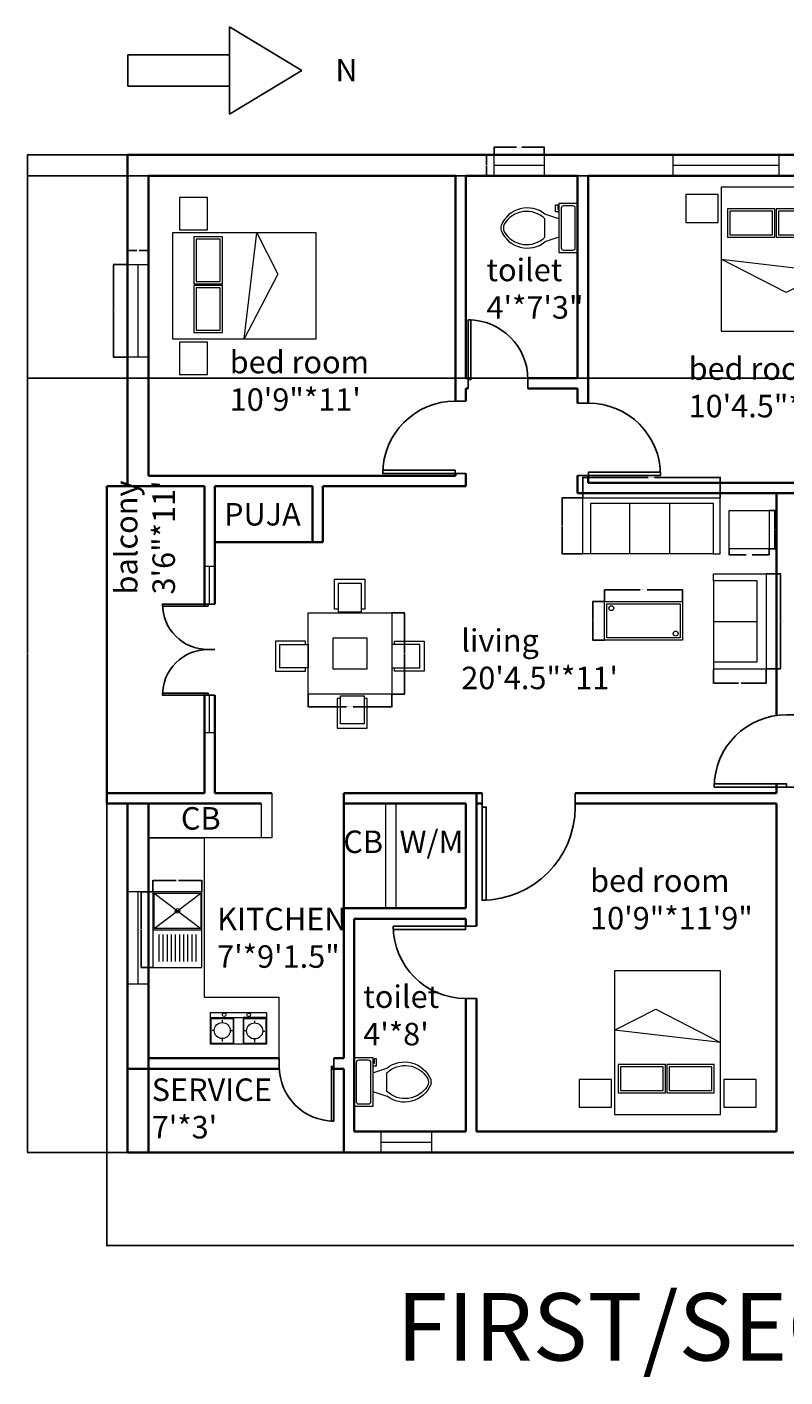
# Model space of a CAD drawing. Units: inches. Extents: x 1632 to 2336, y 1480 to 2095.
# Tile 1 of 2: x 1632 to 1958, y 1480 to 2061. Entities that reach past the tile are written whole.
import ezdxf

# ---------------------------------------------------------------- set-up
doc = ezdxf.new("R2010")
doc.units = ezdxf.units.IN
for name, color, linetype, lineweight in [('A-ANNO-DIMS', 2, 'Continuous', 18), ('A-ANNO-SYMB', 7, 'Continuous', 25), ('A-ANNO-TEXT', 7, 'Continuous', 18), ('A-ANNO-TITL', 7, 'Continuous', 35), ('A-AREA-IDEN', 7, 'Continuous', 18), ('A-DOOR', 3, 'Continuous', 25), ('A-EQPM', 8, 'Continuous', 18), ('A-FLOR-CASE', 9, 'Continuous', 18), ('A-FLOR-FIXT', 9, 'Continuous', 18), ('A-FURN', 8, 'Continuous', 18), ('A-GLAZ', 4, 'Continuous', 18), ('A-WALL', 7, 'Continuous', 35)]:
    doc.layers.add(name, color=color, linetype=linetype, lineweight=lineweight)
doc.styles.get("Standard").update_dxf_attribs({"font": 'arial.ttf'})
doc.dimstyles.get("Standard").update_dxf_attribs({"dimtxt": 0.18, "dimasz": 0.18, "dimexe": 0.18, "dimexo": 0.0625, "dimgap": 0.09, "dimtad": 0, "dimtih": 1, "dimtoh": 1, "dimdec": 4, "dimzin": 0, "dimdsep": 46, "dimtxsty": 'Standard', "dimcen": 0.09, "dimadec": 0, "dimazin": 0, "dimtfac": 1, "dimtdec": 4, "dimtofl": 0, "dimtmove": 0, "dimatfit": 3, "dimfxl": 1, "dimtolj": 1, "dimtzin": 0, "dimarcsym": 0})

# ---------------------------------------------------------------- blocks, each defined once
blk = doc.blocks.new('*U2')
for p, q in [((0, 0), (0, -6)), ((40, 0), (40, -6))]:
    blk.add_line(p, q)
blk.add_lwpolyline([(0, 0), (0, 40), (1.75, 40), (1.75, 0)], close=True)
blk.add_arc((0, 0), 40, 0, 90)
blk = doc.blocks.new('*U4')
for p, q in [((9.5, -6), (9.5, -2)), ((-10, -8.5), (-8, -8.5)), ((-10, -9.5), (-10, -8.5)), ((-7, -9.5), (-10, -9.5)), ((-8, -8.5), (-8, -8)), ((-7, -8), (-7, -9.5)), ((-4, -8), (-6, -14)), ((4, -8), (6, -14)), ((4, -14), (-4, -14))]:
    blk.add_line(p, q)
blk.add_lwpolyline([(10.5, -8), (10.5, 0), (-10.5, 0), (-10.5, -8)], close=True)
for points in [[(-9.5, -2), (-9.5, -6)], [(8.5, -1), (-8.5, -1)], [(-8.5, -7), (8.5, -7)]]:
    blk.add_lwpolyline(points)
for centre, radius, start, end in [((-8.62, -1.88), 0.884, 81.8699, 188.1301), ((8.62, -1.88), 0.884, 351.8699, 98.1301), ((-8.62, -6.12), 0.884, 171.8699, 278.1301), ((8.62, -6.12), 0.884, 261.8699, 8.1301), ((3.52, -21.58), 12.17, 141.46911, 247.97143), ((4.2, -21.82), 11.33, 136.36773, 238.94682), ((-3.52, -21.58), 12.17, 292.02843, 38.53071), ((-4.2, -21.82), 11.33, 301.05301, 43.63209), ((0, -27.88), 4, 245.73182, 294.26817), ((0, -29), 4, 254.86053, 285.13947)]:
    blk.add_arc(centre, radius, start, end)
blk = doc.blocks.new('BED-DOUBLE-WITH-NIGHTSTANDS')
for p, q in [((30.9, 15.3), (36.28, 60.91)), ((36.28, 60.91), (45.27, 43.14)), ((45.27, 43.14), (30.9, 15.3))]:
    blk.add_line(p, q)
for points in [[(3.09, 62.18), (15.1, 62.18), (15.1, 76.08), (3.09, 76.08)], [(0, 15.3), (61.8, 15.3), (61.8, 60.91), (0, 60.91)], [(9.26, 38.94), (21.51, 38.94), (21.51, 59.23), (9.26, 59.23)], [(10.26, 39.94), (20.51, 39.94), (20.51, 58.23), (10.26, 58.23)], [(9.26, 18.02), (21.51, 18.02), (21.51, 38.31), (9.26, 38.31)], [(10.26, 19.02), (20.51, 19.02), (20.51, 37.31), (10.26, 37.31)], [(3.09, 0), (15.1, 0), (15.1, 13.9), (3.09, 13.9)]]:
    blk.add_lwpolyline(points, close=True)
blk = doc.blocks.new('CHAIR-DINING')
for p, q in [((0, 1.12), (0, 13.97)), ((0, 13.97), (12.95, 13.97)), ((12.95, 13.97), (12.95, 1.12)), ((1.47, 1.12), (0, 1.12)), ((12.95, 1.12), (11.55, 1.12))]:
    blk.add_line(p, q)
blk.add_lwpolyline([(1.47, 0), (11.55, 0), (11.55, 12.08), (1.47, 12.08)], close=True)
blk = doc.blocks.new('TABLE-DINING')
for points in [[(0, 35.03), (36, 35.03), (36, 0), (0, 0)], [(10.77, 24.25), (25.23, 24.25), (25.23, 10.77), (10.77, 10.77)]]:
    blk.add_lwpolyline(points, close=True)
blk = doc.blocks.new('SOFA-3-SEAT')
for p, q in [((0, 0), (0, 24.07)), ((0, 24.07), (59, 24.07)), ((59, 0), (59, 24.07)), ((20.13, 21.83), (20.13, 0)), ((37.25, 21.83), (37.25, 0)), ((3.41, 0), (0, 0)), ((56, 0), (59, 0))]:
    blk.add_line(p, q)
blk.add_lwpolyline([(3.41, 21.83), (56, 21.83), (56, 0), (3.41, 0)], close=True)
blk = doc.blocks.new('SOFA-2-SEAT')
for p, q in [((0, 37.84), (0, 40.84)), ((0, 40.84), (22.7, 40.84)), ((22.7, 40.84), (22.7, 0)), ((0, 20.42), (18.79, 20.42)), ((0, 3), (0, 0)), ((0, 0), (22.7, 0))]:
    blk.add_line(p, q)
blk.add_lwpolyline([(18.79, 37.84), (0, 37.84), (0, 3), (18.79, 3)], close=True)
blk = doc.blocks.new('TABLE-COFFEE')
for points in [[(0, 16.65), (33.49, 16.65), (33.49, 0), (0, 0)], [(1, 15.65), (32.49, 15.65), (32.49, 1), (1, 1)]]:
    blk.add_lwpolyline(points, close=True)
for centre in [(2.89, 13.8), (30.54, 2.86)]:
    blk.add_circle(centre, 1.06)
blk = doc.blocks.new('SINK-WITH-DRAINBOARD')
for p, q in [((0.63, 16.78), (20.68, 31.97)), ((0.63, 31.97), (20.68, 16.78)), ((0, 16.25), (21.16, 16.25)), ((2.61, 14.26), (2.61, 2.54)), ((4.39, 14.26), (4.39, 2.54)), ((6.16, 14.26), (6.16, 2.54)), ((7.94, 14.26), (7.94, 2.54)), ((9.72, 14.26), (9.72, 2.54)), ((11.49, 14.26), (11.49, 2.54)), ((13.27, 14.26), (13.27, 2.54)), ((15.04, 14.26), (15.04, 2.54)), ((16.82, 14.26), (16.82, 2.54)), ((18.6, 14.26), (18.6, 2.54))]:
    blk.add_line(p, q)
for points in [[(0, 0), (21.16, 0), (21.16, 32.49), (0, 32.49)], [(0.63, 31.97), (20.68, 31.97), (20.68, 16.78), (0.63, 16.78)]]:
    blk.add_lwpolyline(points, close=True)
blk.add_circle((10.66, 24.37), 0.977)
blk = doc.blocks.new('COOKTOP-2-BURNER')
for p, q in [((0, 11.46), (0, 13.65)), ((0, 13.65), (24.07, 13.65)), ((24.07, 13.65), (24.07, 11.46)), ((0, 11.46), (12, 11.46)), ((0, 11.46), (10, 11.46)), ((1.67, 5.97), (0.82, 5.97)), ((5.23, 9.36), (5.23, 10.33)), ((8.57, 5.88), (9.52, 5.88)), ((10, 11.46), (10, 0)), ((24.07, 11.46), (14.07, 11.46)), ((14.07, 11.46), (14.07, 0)), ((19.15, 9.18), (19.15, 10.15)), ((5.05, 2.47), (5.05, 1.13)), ((15.59, 5.79), (14.74, 5.79)), ((18.97, 2.28), (18.97, 0.95)), ((22.49, 5.7), (23.44, 5.7))]:
    blk.add_line(p, q)
for points in [[(0, 11.46), (24.07, 11.46), (24.07, 0), (0, 0)], [(0.38, 11.07), (9.77, 11.07), (9.77, 0.28), (0.38, 0.28)], [(14.37, 11.14), (23.83, 11.14), (23.83, 0.28), (14.37, 0.28)]]:
    blk.add_lwpolyline(points, close=True)
for centre, radius in [((5.93, 12.7), 0.782), ((16.53, 12.66), 0.782), ((5.12, 5.91), 3.45), ((19.04, 5.73), 3.45)]:
    blk.add_circle(centre, radius)
blk = doc.blocks.new('WINDOW-40')
blk.add_line((4.5, 39.93), (4.5, 0))
blk.add_lwpolyline([(0, 39.93), (9, 39.93), (9, 0), (0, 0)], close=True)
blk = doc.blocks.new('WINDOW-22')
blk.add_line((0, 4.5), (21.58, 4.5))
blk.add_lwpolyline([(0, 9), (21.58, 9), (21.58, 0), (0, 0)], close=True)
blk = doc.blocks.new('WINDOW-45')
blk.add_line((0, 4.5), (45.36, 4.5))
blk.add_lwpolyline([(0, 9), (45.36, 9), (45.36, 0), (0, 0)], close=True)
blk = doc.blocks.new('WINDOW-SIDELIGHT-16')
blk.add_line((2.25, 0), (2.25, 16.22))
blk.add_lwpolyline([(4.5, 0), (0, 0), (0, 16.22), (4.5, 16.22)], close=True)
blk = doc.blocks.new('TABLE-END')
blk.add_lwpolyline([(0, 16.51), (17.12, 16.51), (17.12, 0), (0, 0)], close=True)
blk = doc.blocks.new('COUNTERTOP-L-RETURN')
for p, q in [((0, 94.74), (24, 94.74)), ((24, 94.74), (24, 26.35)), ((24, 26.35), (56.24, 26.35)), ((56.24, 0), (56.24, 26.35))]:
    blk.add_line(p, q)
blk = doc.blocks.new('*D24')
at = {"layer": 'A-ANNO-DIMS', "color": 0, "lineweight": -2, "transparency": 16777216}
for p, q in [((1752.79, 1773.62), (1752.79, 1768.1)), ((1788.79, 1773.62), (1788.79, 1768.1)), ((1752.97, 1768.28), (1769.36, 1768.28)), ((1788.61, 1768.28), (1772.23, 1768.28))]:
    blk.add_line(p, q, dxfattribs=at)
at = {"layer": 'A-ANNO-DIMS', "color": 0, "transparency": 16777216}
for points in [[(1752.97, 1768.31), (1752.97, 1768.25), (1752.79, 1768.28)], [(1788.61, 1768.31), (1788.61, 1768.25), (1788.79, 1768.28)]]:
    blk.add_solid(points, dxfattribs=at)
at = {"layer": 'Defpoints', "color": 0, "transparency": 16777216}
for p in [(1752.79, 1773.69), (1788.79, 1773.69), (1788.79, 1768.28)]:
    blk.add_point(p, dxfattribs=at)
at = {"layer": 'A-ANNO-DIMS', "color": 0, "transparency": 16777216, "insert": (1770.79, 1768.28), "char_height": 0.18, "attachment_point": 5}
blk.add_mtext('\\A1;DINING TABLE 36 TYP.', dxfattribs=at)
blk = doc.blocks.new('*D25')
at = {"layer": 'A-ANNO-DIMS', "color": 0, "lineweight": -2, "transparency": 16777216}
for p, q in [((1788.86, 1808.71), (1794.37, 1808.71)), ((1794.19, 1808.53), (1794.19, 1791.38)), ((1794.19, 1773.87), (1794.19, 1791.02)), ((1788.86, 1773.69), (1794.37, 1773.69))]:
    blk.add_line(p, q, dxfattribs=at)
at = {"layer": 'A-ANNO-DIMS', "color": 0, "transparency": 16777216}
for points in [[(1794.16, 1808.53), (1794.22, 1808.53), (1794.19, 1808.71)], [(1794.16, 1773.87), (1794.22, 1773.87), (1794.19, 1773.69)]]:
    blk.add_solid(points, dxfattribs=at)
at = {"layer": 'Defpoints', "color": 0, "transparency": 16777216}
for p in [(1788.79, 1808.71), (1794.19, 1808.71), (1788.79, 1773.69)]:
    blk.add_point(p, dxfattribs=at)
at = {"layer": 'A-ANNO-DIMS', "color": 0, "transparency": 16777216, "insert": (1794.19, 1791.2), "char_height": 0.18, "attachment_point": 5}
blk.add_mtext('\\A1;35 TYP.', dxfattribs=at)
blk = doc.blocks.new('*D26')
at = {"layer": 'A-ANNO-DIMS', "color": 0, "lineweight": -2, "transparency": 16777216}
for p, q in [((1870.91, 1858.14), (1870.91, 1867.11)), ((1871.09, 1866.93), (1899.03, 1866.93)), ((1929.73, 1866.93), (1901.79, 1866.93)), ((1929.91, 1858.14), (1929.91, 1867.11))]:
    blk.add_line(p, q, dxfattribs=at)
at = {"layer": 'A-ANNO-DIMS', "color": 0, "transparency": 16777216}
for points in [[(1871.09, 1866.96), (1871.09, 1866.9), (1870.91, 1866.93)], [(1929.73, 1866.96), (1929.73, 1866.9), (1929.91, 1866.93)]]:
    blk.add_solid(points, dxfattribs=at)
at = {"layer": 'Defpoints', "color": 0, "transparency": 16777216}
for p in [(1929.91, 1866.93), (1870.91, 1858.08), (1929.91, 1858.08)]:
    blk.add_point(p, dxfattribs=at)
at = {"layer": 'A-ANNO-DIMS', "color": 0, "transparency": 16777216, "insert": (1900.41, 1866.93), "char_height": 0.18, "attachment_point": 5}
blk.add_mtext('\\A1;3-SEAT SOFA 59 TYP.', dxfattribs=at)
blk = doc.blocks.new('*D27')
at = {"layer": 'A-ANNO-DIMS', "color": 0, "lineweight": -2, "transparency": 16777216}
for p, q in [((1870.85, 1858.08), (1861.88, 1858.08)), ((1862.06, 1857.9), (1862.06, 1846.22)), ((1862.06, 1834.18), (1862.06, 1845.86)), ((1870.85, 1834), (1861.88, 1834))]:
    blk.add_line(p, q, dxfattribs=at)
at = {"layer": 'A-ANNO-DIMS', "color": 0, "transparency": 16777216}
for points in [[(1862.03, 1857.9), (1862.09, 1857.9), (1862.06, 1858.08)], [(1862.03, 1834.18), (1862.09, 1834.18), (1862.06, 1834)]]:
    blk.add_solid(points, dxfattribs=at)
at = {"layer": 'Defpoints', "color": 0, "transparency": 16777216}
for p in [(1862.06, 1858.08), (1870.91, 1858.08), (1870.91, 1834)]:
    blk.add_point(p, dxfattribs=at)
at = {"layer": 'A-ANNO-DIMS', "color": 0, "transparency": 16777216, "insert": (1862.06, 1846.04), "char_height": 0.18, "attachment_point": 5}
blk.add_mtext('\\A1;24 TYP.', dxfattribs=at)
blk = doc.blocks.new('*D28')
at = {"layer": 'A-ANNO-DIMS', "color": 0, "lineweight": -2, "transparency": 16777216}
for p, q in [((1949.81, 1825.39), (1956.05, 1825.39)), ((1955.87, 1825.21), (1955.87, 1805.15)), ((1955.87, 1784.73), (1955.87, 1804.79)), ((1949.81, 1784.55), (1956.05, 1784.55))]:
    blk.add_line(p, q, dxfattribs=at)
at = {"layer": 'A-ANNO-DIMS', "color": 0, "transparency": 16777216}
for points in [[(1955.84, 1825.21), (1955.9, 1825.21), (1955.87, 1825.39)], [(1955.84, 1784.73), (1955.9, 1784.73), (1955.87, 1784.55)]]:
    blk.add_solid(points, dxfattribs=at)
at = {"layer": 'Defpoints', "color": 0, "transparency": 16777216}
for p in [(1949.74, 1825.39), (1955.87, 1825.39), (1949.74, 1784.55)]:
    blk.add_point(p, dxfattribs=at)
at = {"layer": 'A-ANNO-DIMS', "color": 0, "transparency": 16777216, "insert": (1955.87, 1804.97), "char_height": 0.18, "attachment_point": 5}
blk.add_mtext('\\A1;2-SEAT SOFA 41 TYP.', dxfattribs=at)
blk = doc.blocks.new('*D29')
at = {"layer": 'A-ANNO-DIMS', "color": 0, "lineweight": -2, "transparency": 16777216}
for p, q in [((1927.05, 1784.49), (1927.05, 1778.24)), ((1949.74, 1784.49), (1949.74, 1778.24)), ((1927.23, 1778.42), (1937.87, 1778.42)), ((1949.56, 1778.42), (1938.93, 1778.42))]:
    blk.add_line(p, q, dxfattribs=at)
at = {"layer": 'A-ANNO-DIMS', "color": 0, "transparency": 16777216}
for points in [[(1927.23, 1778.45), (1927.23, 1778.39), (1927.05, 1778.42)], [(1949.56, 1778.45), (1949.56, 1778.39), (1949.74, 1778.42)]]:
    blk.add_solid(points, dxfattribs=at)
at = {"layer": 'Defpoints', "color": 0, "transparency": 16777216}
for p in [(1927.05, 1784.55), (1949.74, 1784.55), (1949.74, 1778.42)]:
    blk.add_point(p, dxfattribs=at)
at = {"layer": 'A-ANNO-DIMS', "color": 0, "transparency": 16777216, "insert": (1938.4, 1778.42), "char_height": 0.18, "attachment_point": 5}
blk.add_mtext('\\A1;23 TYP.', dxfattribs=at)
blk = doc.blocks.new('*D30')
at = {"layer": 'A-ANNO-DIMS', "color": 0, "lineweight": -2, "transparency": 16777216}
for p, q in [((1933.85, 1836.1), (1933.85, 1833.42)), ((1950.97, 1836.1), (1950.97, 1833.42)), ((1934.03, 1833.6), (1941.15, 1833.6)), ((1950.79, 1833.6), (1943.67, 1833.6))]:
    blk.add_line(p, q, dxfattribs=at)
at = {"layer": 'A-ANNO-DIMS', "color": 0, "transparency": 16777216}
for points in [[(1934.03, 1833.63), (1934.03, 1833.57), (1933.85, 1833.6)], [(1950.79, 1833.63), (1950.79, 1833.57), (1950.97, 1833.6)]]:
    blk.add_solid(points, dxfattribs=at)
at = {"layer": 'Defpoints', "color": 0, "transparency": 16777216}
for p in [(1933.85, 1836.17), (1950.97, 1836.17), (1950.97, 1833.6)]:
    blk.add_point(p, dxfattribs=at)
at = {"layer": 'A-ANNO-DIMS', "color": 0, "transparency": 16777216, "insert": (1942.41, 1833.6), "char_height": 0.18, "attachment_point": 5}
blk.add_mtext('\\A1;END TABLE 17 TYP.', dxfattribs=at)
blk = doc.blocks.new('*D31')
at = {"layer": 'A-ANNO-DIMS', "color": 0, "lineweight": -2, "transparency": 16777216}
for p, q in [((1951.03, 1852.67), (1953.72, 1852.67)), ((1953.54, 1852.49), (1953.54, 1844.6)), ((1953.54, 1836.35), (1953.54, 1844.24)), ((1951.03, 1836.17), (1953.72, 1836.17))]:
    blk.add_line(p, q, dxfattribs=at)
at = {"layer": 'A-ANNO-DIMS', "color": 0, "transparency": 16777216}
for points in [[(1953.51, 1852.49), (1953.57, 1852.49), (1953.54, 1852.67)], [(1953.51, 1836.35), (1953.57, 1836.35), (1953.54, 1836.17)]]:
    blk.add_solid(points, dxfattribs=at)
at = {"layer": 'Defpoints', "color": 0, "transparency": 16777216}
for p in [(1950.97, 1852.67), (1953.54, 1852.67), (1950.97, 1836.17)]:
    blk.add_point(p, dxfattribs=at)
at = {"layer": 'A-ANNO-DIMS', "color": 0, "transparency": 16777216, "insert": (1953.54, 1844.42), "char_height": 0.18, "attachment_point": 5}
blk.add_mtext('\\A1;17 TYP.', dxfattribs=at)
blk = doc.blocks.new('*D32')
at = {"layer": 'A-ANNO-DIMS', "color": 0, "lineweight": -2, "transparency": 16777216}
for p, q in [((1880.29, 1813.6), (1880.29, 1818.74)), ((1880.47, 1818.56), (1895.53, 1818.56)), ((1913.6, 1818.56), (1898.54, 1818.56)), ((1913.78, 1813.6), (1913.78, 1818.74))]:
    blk.add_line(p, q, dxfattribs=at)
at = {"layer": 'A-ANNO-DIMS', "color": 0, "transparency": 16777216}
for points in [[(1880.47, 1818.59), (1880.47, 1818.53), (1880.29, 1818.56)], [(1913.6, 1818.59), (1913.6, 1818.53), (1913.78, 1818.56)]]:
    blk.add_solid(points, dxfattribs=at)
at = {"layer": 'Defpoints', "color": 0, "transparency": 16777216}
for p in [(1913.78, 1818.56), (1880.29, 1813.54), (1913.78, 1813.54)]:
    blk.add_point(p, dxfattribs=at)
at = {"layer": 'A-ANNO-DIMS', "color": 0, "transparency": 16777216, "insert": (1897.03, 1818.56), "char_height": 0.18, "attachment_point": 5}
blk.add_mtext('\\A1;COFFEE TABLE 33 TYP.', dxfattribs=at)
blk = doc.blocks.new('*D33')
at = {"layer": 'A-ANNO-DIMS', "color": 0, "lineweight": -2, "transparency": 16777216}
for p, q in [((1880.23, 1813.54), (1875.09, 1813.54)), ((1875.27, 1813.36), (1875.27, 1805.39)), ((1875.27, 1797.07), (1875.27, 1805.03)), ((1880.23, 1796.89), (1875.09, 1796.89))]:
    blk.add_line(p, q, dxfattribs=at)
at = {"layer": 'A-ANNO-DIMS', "color": 0, "transparency": 16777216}
for points in [[(1875.24, 1813.36), (1875.3, 1813.36), (1875.27, 1813.54)], [(1875.24, 1797.07), (1875.3, 1797.07), (1875.27, 1796.89)]]:
    blk.add_solid(points, dxfattribs=at)
at = {"layer": 'Defpoints', "color": 0, "transparency": 16777216}
for p in [(1875.27, 1813.54), (1880.29, 1813.54), (1880.29, 1796.89)]:
    blk.add_point(p, dxfattribs=at)
at = {"layer": 'A-ANNO-DIMS', "color": 0, "transparency": 16777216, "insert": (1875.27, 1805.21), "char_height": 0.18, "attachment_point": 5}
blk.add_mtext('\\A1;17 TYP.', dxfattribs=at)
blk = doc.blocks.new('*D34')
at = {"layer": 'A-ANNO-DIMS', "color": 0, "lineweight": -2, "transparency": 16777216}
for p, q in [((1675.09, 1958.49), (1668.98, 1958.49)), ((1669.16, 1958.31), (1669.16, 1938.71)), ((1669.16, 1918.74), (1669.16, 1938.34)), ((1675.09, 1918.56), (1668.98, 1918.56))]:
    blk.add_line(p, q, dxfattribs=at)
at = {"layer": 'A-ANNO-DIMS', "color": 0, "transparency": 16777216}
for points in [[(1669.13, 1958.31), (1669.19, 1958.31), (1669.16, 1958.49)], [(1669.13, 1918.74), (1669.19, 1918.74), (1669.16, 1918.56)]]:
    blk.add_solid(points, dxfattribs=at)
at = {"layer": 'Defpoints', "color": 0, "transparency": 16777216}
for p in [(1669.16, 1958.49), (1675.15, 1958.49), (1675.15, 1918.56)]:
    blk.add_point(p, dxfattribs=at)
at = {"layer": 'A-ANNO-DIMS', "color": 0, "transparency": 16777216, "insert": (1669.16, 1938.52), "char_height": 0.18, "attachment_point": 5}
blk.add_mtext('\\A1;WINDOW 40 TYP.', dxfattribs=at)
blk = doc.blocks.new('*D35')
at = {"layer": 'A-ANNO-DIMS', "color": 0, "lineweight": -2, "transparency": 16777216}
for p, q in [((1675.15, 1958.55), (1675.15, 1964.66)), ((1675.33, 1964.48), (1679.19, 1964.48)), ((1683.97, 1964.48), (1680.11, 1964.48)), ((1684.15, 1958.55), (1684.15, 1964.66))]:
    blk.add_line(p, q, dxfattribs=at)
at = {"layer": 'A-ANNO-DIMS', "color": 0, "transparency": 16777216}
for points in [[(1675.33, 1964.51), (1675.33, 1964.45), (1675.15, 1964.48)], [(1683.97, 1964.51), (1683.97, 1964.45), (1684.15, 1964.48)]]:
    blk.add_solid(points, dxfattribs=at)
at = {"layer": 'Defpoints', "color": 0, "transparency": 16777216}
for p in [(1684.15, 1964.48), (1675.15, 1958.49), (1684.15, 1958.49)]:
    blk.add_point(p, dxfattribs=at)
at = {"layer": 'A-ANNO-DIMS', "color": 0, "transparency": 16777216, "insert": (1679.65, 1964.48), "char_height": 0.18, "attachment_point": 5}
blk.add_mtext('\\A1;9 TYP.', dxfattribs=at)
blk = doc.blocks.new('*D36')
at = {"layer": 'A-ANNO-DIMS', "color": 0, "lineweight": -2, "transparency": 16777216}
for p, q in [((1832.78, 2005.69), (1832.78, 2009.04)), ((1832.96, 2008.86), (1842.46, 2008.86)), ((1854.18, 2008.86), (1844.69, 2008.86)), ((1854.36, 2005.69), (1854.36, 2009.04))]:
    blk.add_line(p, q, dxfattribs=at)
at = {"layer": 'A-ANNO-DIMS', "color": 0, "transparency": 16777216}
for points in [[(1832.96, 2008.89), (1832.96, 2008.83), (1832.78, 2008.86)], [(1854.18, 2008.89), (1854.18, 2008.83), (1854.36, 2008.86)]]:
    blk.add_solid(points, dxfattribs=at)
at = {"layer": 'Defpoints', "color": 0, "transparency": 16777216}
for p in [(1854.36, 2008.86), (1832.78, 2005.62), (1854.36, 2005.62)]:
    blk.add_point(p, dxfattribs=at)
at = {"layer": 'A-ANNO-DIMS', "color": 0, "transparency": 16777216, "insert": (1843.57, 2008.86), "char_height": 0.18, "attachment_point": 5}
blk.add_mtext('\\A1;WINDOW 22 TYP.', dxfattribs=at)
blk = doc.blocks.new('*D37')
at = {"layer": 'A-ANNO-DIMS', "color": 0, "lineweight": -2, "transparency": 16777216}
for p, q in [((1832.72, 2005.62), (1829.37, 2005.62)), ((1829.55, 2005.44), (1829.55, 2001.31)), ((1829.55, 1996.8), (1829.55, 2000.94)), ((1832.72, 1996.62), (1829.37, 1996.62))]:
    blk.add_line(p, q, dxfattribs=at)
at = {"layer": 'A-ANNO-DIMS', "color": 0, "transparency": 16777216}
for points in [[(1829.52, 2005.44), (1829.58, 2005.44), (1829.55, 2005.62)], [(1829.52, 1996.8), (1829.58, 1996.8), (1829.55, 1996.62)]]:
    blk.add_solid(points, dxfattribs=at)
at = {"layer": 'Defpoints', "color": 0, "transparency": 16777216}
for p in [(1829.55, 2005.62), (1832.78, 2005.62), (1832.78, 1996.62)]:
    blk.add_point(p, dxfattribs=at)
at = {"layer": 'A-ANNO-DIMS', "color": 0, "transparency": 16777216, "insert": (1829.55, 2001.12), "char_height": 0.18, "attachment_point": 5}
blk.add_mtext('\\A1;9 TYP.', dxfattribs=at)
blk = doc.blocks.new('*D42')
at = {"layer": 'A-ANNO-DIMS', "color": 0, "lineweight": -2, "transparency": 16777216}
for p, q in [((1685.91, 1688.67), (1680.92, 1688.67)), ((1681.1, 1688.49), (1681.1, 1672.6)), ((1681.1, 1656.35), (1681.1, 1672.24)), ((1685.91, 1656.17), (1680.92, 1656.17))]:
    blk.add_line(p, q, dxfattribs=at)
at = {"layer": 'A-ANNO-DIMS', "color": 0, "transparency": 16777216}
for points in [[(1681.07, 1688.49), (1681.13, 1688.49), (1681.1, 1688.67)], [(1681.07, 1656.35), (1681.13, 1656.35), (1681.1, 1656.17)]]:
    blk.add_solid(points, dxfattribs=at)
at = {"layer": 'Defpoints', "color": 0, "transparency": 16777216}
for p in [(1681.1, 1688.67), (1685.98, 1688.67), (1685.98, 1656.17)]:
    blk.add_point(p, dxfattribs=at)
at = {"layer": 'A-ANNO-DIMS', "color": 0, "transparency": 16777216, "insert": (1681.1, 1672.42), "char_height": 0.18, "attachment_point": 5}
blk.add_mtext('\\A1;SINK 32 TYP.', dxfattribs=at)
blk = doc.blocks.new('*D43')
at = {"layer": 'A-ANNO-DIMS', "color": 0, "lineweight": -2, "transparency": 16777216}
for p, q in [((1685.98, 1688.73), (1685.98, 1693.72)), ((1686.16, 1693.54), (1696.02, 1693.54)), ((1706.95, 1693.54), (1697.08, 1693.54)), ((1707.13, 1688.73), (1707.13, 1693.72))]:
    blk.add_line(p, q, dxfattribs=at)
at = {"layer": 'A-ANNO-DIMS', "color": 0, "transparency": 16777216}
for points in [[(1686.16, 1693.57), (1686.16, 1693.51), (1685.98, 1693.54)], [(1706.95, 1693.57), (1706.95, 1693.51), (1707.13, 1693.54)]]:
    blk.add_solid(points, dxfattribs=at)
at = {"layer": 'Defpoints', "color": 0, "transparency": 16777216}
for p in [(1707.13, 1693.54), (1685.98, 1688.67), (1707.13, 1688.67)]:
    blk.add_point(p, dxfattribs=at)
at = {"layer": 'A-ANNO-DIMS', "color": 0, "transparency": 16777216, "insert": (1696.55, 1693.54), "char_height": 0.18, "attachment_point": 5}
blk.add_mtext('\\A1;21 TYP.', dxfattribs=at)
blk = doc.blocks.new('*D48')
at = {"layer": 'A-ANNO-DIMS', "color": 0, "lineweight": -2, "transparency": 16777216}
for p, q in [((1666.2, 1731.06), (1666.2, 1536.39)), ((2335.15, 1728.06), (2335.15, 1536.39)), ((1666.38, 1536.57), (2000.39, 1536.57)), ((2334.97, 1536.57), (2000.97, 1536.57))]:
    blk.add_line(p, q, dxfattribs=at)
at = {"layer": 'A-ANNO-DIMS', "color": 0, "transparency": 16777216}
for points in [[(1666.38, 1536.6), (1666.38, 1536.54), (1666.2, 1536.57)], [(2334.97, 1536.6), (2334.97, 1536.54), (2335.15, 1536.57)]]:
    blk.add_solid(points, dxfattribs=at)
at = {"layer": 'Defpoints', "color": 0, "transparency": 16777216}
for p in [(1666.2, 1731.12), (2335.15, 1728.12), (2335.15, 1536.57)]:
    blk.add_point(p, dxfattribs=at)
at = {"layer": 'A-ANNO-DIMS', "color": 0, "transparency": 16777216, "insert": (2000.68, 1536.57), "char_height": 0.18, "attachment_point": 5}
blk.add_mtext('\\A1;669', dxfattribs=at)
blk = doc.blocks.new('*D49')
at = {"layer": 'A-ANNO-DIMS', "color": 0, "lineweight": -2, "transparency": 16777216}
for p, q in [((1675.09, 2005.62), (1631.97, 2005.62)), ((1632.15, 2005.44), (1632.15, 1791.31)), ((1632.15, 1576.8), (1632.15, 1790.94)), ((1675.09, 1576.62), (1631.97, 1576.62))]:
    blk.add_line(p, q, dxfattribs=at)
at = {"layer": 'A-ANNO-DIMS', "color": 0, "transparency": 16777216}
for points in [[(1632.12, 2005.44), (1632.18, 2005.44), (1632.15, 2005.62)], [(1632.12, 1576.8), (1632.18, 1576.8), (1632.15, 1576.62)]]:
    blk.add_solid(points, dxfattribs=at)
at = {"layer": 'Defpoints', "color": 0, "transparency": 16777216}
for p in [(1632.15, 2005.62), (1675.15, 2005.62), (1675.15, 1576.62)]:
    blk.add_point(p, dxfattribs=at)
at = {"layer": 'A-ANNO-DIMS', "color": 0, "transparency": 16777216, "insert": (1632.15, 1791.12), "char_height": 0.18, "attachment_point": 5}
blk.add_mtext('\\A1;429', dxfattribs=at)
blk = doc.blocks.new('*D52')
at = {"layer": 'A-ANNO-DIMS', "color": 0, "lineweight": -2, "transparency": 16777216}
for p, q in [((2188.09, 1996.62), (1631.97, 1996.62)), ((1632.15, 1996.44), (1632.15, 1953.31)), ((1632.15, 1909.8), (1632.15, 1952.94)), ((2188.09, 1909.62), (1631.97, 1909.62))]:
    blk.add_line(p, q, dxfattribs=at)
at = {"layer": 'A-ANNO-DIMS', "color": 0, "transparency": 16777216}
for points in [[(1632.12, 1996.44), (1632.18, 1996.44), (1632.15, 1996.62)], [(1632.12, 1909.8), (1632.18, 1909.8), (1632.15, 1909.62)]]:
    blk.add_solid(points, dxfattribs=at)
at = {"layer": 'Defpoints', "color": 0, "transparency": 16777216}
for p in [(1632.15, 1996.62), (2188.15, 1996.62), (2188.15, 1909.62)]:
    blk.add_point(p, dxfattribs=at)
at = {"layer": 'A-ANNO-DIMS', "color": 0, "transparency": 16777216, "insert": (1632.15, 1953.12), "char_height": 0.18, "attachment_point": 5}
blk.add_mtext('\\A1;87', dxfattribs=at)

msp = doc.modelspace()

# ---------------------------------------------------------------- linework, layer by layer
at = {"layer": 'A-ANNO-SYMB'}
for p, q in [((1718.97, 2048.58), (1718.97, 2060.58)), ((1718.97, 2060.58), (1750.16, 2041.85)), ((1718.97, 2023.13), (1750.16, 2041.85)), ((1718.97, 2035.13), (1718.97, 2023.13))]:
    msp.add_line(p, q, dxfattribs=at)
msp.add_lwpolyline([(1675.31, 2035.13), (1718.97, 2035.13), (1718.97, 2048.58), (1675.31, 2048.58)], close=True, dxfattribs=at)
at = {"layer": 'A-FLOR-CASE'}
for p, q in [((1737.15, 1731.12), (1737.15, 1711.87)), ((1732.65, 1726.62), (1732.65, 1711.87)), ((1786.07, 1726.62), (1786.07, 1681.62)), ((1790.57, 1726.62), (1790.57, 1681.62)), ((1737.15, 1711.87), (1684.15, 1711.87))]:
    msp.add_line(p, q, dxfattribs=at)
at = {"layer": 'A-WALL'}
for p, q in [((1675.15, 2005.62), (1820.65, 2005.62)), ((1675.15, 1863.12), (1675.15, 2005.62)), ((1820.65, 2005.62), (1873.15, 2005.62)), ((1873.15, 2005.62), (2006.65, 2005.62)), ((1684.15, 1996.62), (1816.15, 1996.62)), ((1684.15, 1867.62), (1684.15, 1996.62)), ((1816.15, 1996.62), (1816.15, 1899.69)), ((1820.65, 1996.62), (1820.65, 1909.62)), ((1820.65, 1996.62), (1868.65, 1996.62)), ((1868.65, 1996.62), (1868.65, 1909.62)), ((1873.15, 1996.62), (1873.15, 1905.12)), ((1873.15, 1996.62), (1997.65, 1996.62)), ((1822.81, 1909.62), (1820.65, 1909.62)), ((1820.65, 1905.12), (1820.65, 1899.69)), ((1821.68, 1905.12), (1820.65, 1905.12)), ((1868.65, 1909.62), (1847.31, 1909.62)), ((1868.65, 1905.12), (1847.32, 1905.12)), ((1868.65, 1905.12), (1868.65, 1898.84)), ((1873.15, 1898.84), (1873.15, 1905.12)), ((1816.15, 1867.62), (1684.15, 1867.62)), ((1816.15, 1868.62), (1816.15, 1867.62)), ((1820.65, 1868.62), (1820.65, 1863.12)), ((1868.65, 1867.77), (1868.65, 1860.12)), ((1873.15, 1864.62), (1873.15, 1867.77)), ((1997.65, 1864.62), (1873.15, 1864.62)), ((1666.2, 1726.62), (1666.2, 1863.12)), ((1666.2, 1863.12), (1672.2, 1863.12)), ((1672.2, 1863.12), (1708.2, 1863.12)), ((1708.2, 1863.12), (1675.15, 1863.12)), ((1708.2, 1863.12), (1708.2, 1811.62)), ((1712.7, 1863.12), (1712.7, 1812.47)), ((1712.7, 1863.12), (1754.7, 1863.12)), ((1712.7, 1863.12), (1754.7, 1863.12)), ((1754.7, 1863.12), (1712.7, 1863.12)), ((1754.7, 1863.12), (1754.7, 1839.12)), ((1820.65, 1863.12), (1759.2, 1863.12)), ((1759.2, 1863.12), (1759.2, 1839.12)), ((1759.2, 1863.12), (1772.7, 1863.12)), ((1997.65, 1860.12), (1868.65, 1860.12)), ((1954.15, 1845.35), (1954.15, 1860.12)), ((1954.15, 1845.35), (1954.15, 1776.35)), ((1759.2, 1839.12), (1712.7, 1839.12)), ((1708.2, 1792.96), (1708.2, 1792.83)), ((1954.15, 1776.35), (1954.15, 1764.54)), ((1708.2, 1774.18), (1708.2, 1731.12)), ((1712.7, 1773.32), (1712.7, 1731.12)), ((1708.2, 1731.12), (1666.2, 1731.12)), ((1737.15, 1731.12), (1712.7, 1731.12)), ((1825.15, 1731.12), (1768.15, 1731.12)), ((1768.15, 1726.62), (1768.15, 1731.12)), ((1827.62, 1731.12), (1825.15, 1731.12)), ((1825.15, 1673.94), (1825.15, 1731.12)), ((1954.15, 1731.12), (1867.62, 1731.12)), ((1954.15, 1735.14), (1954.15, 1731.12)), ((1712.7, 1726.62), (1666.2, 1726.62)), ((1675.15, 1726.62), (1675.15, 1612.62)), ((1684.15, 1726.62), (1684.15, 1617.12)), ((1732.65, 1726.62), (1712.7, 1726.62)), ((1768.15, 1617.12), (1768.15, 1726.62)), ((1772.65, 1726.62), (1768.15, 1726.62)), ((1820.65, 1726.62), (1772.65, 1726.62)), ((1820.65, 1681.62), (1820.65, 1726.62)), ((1827.62, 1726.62), (1825.15, 1726.62)), ((1954.15, 1726.62), (1867.62, 1726.62)), ((1954.15, 1585.62), (1954.15, 1726.62)), ((1772.65, 1681.62), (1768.15, 1681.62)), ((1777.15, 1681.62), (1772.65, 1681.62)), ((1820.65, 1681.62), (1777.15, 1681.62)), ((1772.65, 1612.62), (1772.65, 1677.12)), ((1777.15, 1677.12), (1772.65, 1677.12)), ((1820.65, 1677.12), (1777.15, 1677.12)), ((1820.65, 1673.94), (1820.65, 1677.12)), ((1820.65, 1585.62), (1820.65, 1642.88)), ((1825.15, 1585.62), (1825.15, 1642.88)), ((1825.15, 1585.62), (1825.15, 1642.88)), ((1684.15, 1612.62), (1684.15, 1631.26)), ((1684.15, 1617.12), (1740.39, 1617.12)), ((1763.84, 1617.12), (1768.15, 1617.12)), ((1675.15, 1612.62), (1740.42, 1612.62)), ((1675.15, 1612.62), (1675.15, 1576.62)), ((1684.15, 1612.62), (1684.15, 1576.62)), ((1762.81, 1612.62), (1768.15, 1612.62)), ((1768.15, 1576.62), (1768.15, 1612.62)), ((1772.65, 1585.62), (1772.65, 1612.62)), ((1772.65, 1585.62), (1820.65, 1585.62)), ((1825.15, 1585.62), (1954.15, 1585.62)), ((1675.15, 1576.62), (1772.65, 1576.62)), ((1684.15, 1576.62), (1768.15, 1576.62)), ((1772.65, 1576.62), (1825.15, 1576.62)), ((1825.15, 1576.62), (1963.15, 1576.62))]:
    msp.add_line(p, q, dxfattribs=at)

# ---------------------------------------------------------------- block references
at = {"layer": 'A-DOOR', "xscale": 0.6408249326853631, "yscale": 0.6408249326853631, "zscale": 0.6408249326853631}
msp.add_blockref('*U2', (1821.68, 1908.97), dxfattribs=at)
at = {"layer": 'A-DOOR'}
for p, xscale, yscale, zscale, rotation in [((1815.99, 1868.62), 0.7765731612885453, 0.7765731612885453, 0.7765731612885453, 90), ((1873.31, 1867.77), -0.7765731612885453, 0.7765731612885453, 0.7765731612885453, 270), ((1709.77, 1812.47), -0.4894447198564081, 0.4894447198564081, 0.4894447198564081, 90), ((1709.77, 1773.32), 0.4894447198564081, 0.4894447198564081, 0.4894447198564081, 89.99999999999999), ((1958.49, 1733.78), 0.7765731612885453, 0.7765731612885453, 0.7765731612885453, 90), ((1820.49, 1673.94), -0.7765731612885453, 0.7765731612885453, 0.7765731612885453, 90), ((1763.84, 1613.61), 0.5860402873761541, 0.5860402873761541, 0.5860402873761541, 180)]:
    msp.add_blockref('*U2', p, dxfattribs=dict(at, xscale=xscale, yscale=yscale, zscale=zscale, rotation=rotation))
at = {"layer": 'A-DOOR', "xscale": -1, "rotation": 180}
msp.add_blockref('*U2', (1827.62, 1725.12), dxfattribs=at)
at = {"layer": 'A-EQPM'}
msp.add_blockref('COOKTOP-2-BURNER', (1710.78, 1623.16), dxfattribs=at)
at = {"layer": 'A-FLOR-CASE'}
msp.add_blockref('COUNTERTOP-L-RETURN', (1684.15, 1617.12), dxfattribs=at)
at = {"layer": 'A-FLOR-FIXT', "rotation": 270}
msp.add_blockref('*U4', (1868.65, 1974.15), dxfattribs=at)
at = {"layer": 'A-FLOR-FIXT'}
msp.add_blockref('SINK-WITH-DRAINBOARD', (1685.98, 1656.17), dxfattribs=at)
at = {"layer": 'A-FLOR-FIXT', "xscale": -1, "rotation": 90}
msp.add_blockref('*U4', (1772.65, 1606.91), dxfattribs=at)
at = {"layer": 'A-FURN'}
for name, p, rotation in [('BED-DOUBLE-WITH-NIGHTSTANDS', (1915.16, 1991.66), 269.9999999999999), ('CHAIR-DINING', (1788.79, 1796.52), 269.9999999999956), ('BED-DOUBLE-WITH-NIGHTSTANDS', (1945.4, 1592.96), 89.99999999999909)]:
    msp.add_blockref(name, p, dxfattribs=dict(at, rotation=rotation))
for name, p in [('BED-DOUBLE-WITH-NIGHTSTANDS', (1694.48, 1911.14)), ('SOFA-3-SEAT', (1870.91, 1834)), ('TABLE-END', (1933.85, 1836.16)), ('CHAIR-DINING', (1764.2, 1809.16)), ('SOFA-2-SEAT', (1927.05, 1784.55)), ('TABLE-COFFEE', (1880.29, 1796.89)), ('TABLE-DINING', (1752.79, 1773.68))]:
    msp.add_blockref(name, p, dxfattribs=at)
at = {"layer": 'A-FURN', "extrusion": (0, 0, -1), "zscale": -1}
for p, rotation in [((-1752.79, 1796.52), 269.9999999999933), ((-1765.3, 1773.02), 180)]:
    msp.add_blockref('CHAIR-DINING', p, dxfattribs=dict(at, rotation=rotation))
at = {"layer": 'A-GLAZ'}
for name, p in [('WINDOW-22', (1832.78, 1996.62)), ('WINDOW-45', (1909.82, 1996.62)), ('WINDOW-40', (1675.15, 1918.56)), ('WINDOW-SIDELIGHT-16', (1708.2, 1812.47)), ('WINDOW-SIDELIGHT-16', (1708.2, 1757.1)), ('WINDOW-40', (1675.15, 1648.99)), ('WINDOW-22', (1784.28, 1576.62))]:
    msp.add_blockref(name, p, dxfattribs=at)

# ---------------------------------------------------------------- texts
at = {"layer": 'A-ANNO-SYMB', "insert": (1764.54, 2046.88), "char_height": 9.67, "attachment_point": 1}
msp.add_mtext_dynamic_manual_height_columns('N', width=166.6207, gutter_width=48.36, heights=[0], dxfattribs=at)
at = {"layer": 'A-ANNO-TEXT', "char_height": 9.673, "attachment_point": 1}
for s, insert in [('CB', (1698.12, 1725.14)), ('CB', (1767.94, 1715.06)), ('W/M', (1792.12, 1715.06))]:
    msp.add_mtext_dynamic_manual_height_columns(s, width=166.6207, gutter_width=48.36, heights=[0], dxfattribs=dict(at, insert=insert))
at = {"layer": 'A-ANNO-TITL', "insert": (1790.83, 1516.15), "char_height": 28.9764, "attachment_point": 1}
msp.add_mtext_dynamic_manual_height_columns('FIRST/SECOND FLOOR', width=499.1431, gutter_width=144.88, heights=[77.88], dxfattribs=at)
at = {"layer": 'A-AREA-IDEN', "attachment_point": 1}
for s, insert, char_height in [('toilet\\P4\'*7\'3"', (1829.49, 1960.96), 9.673), ('bed room\\P10\'9"*11\'', (1719.09, 1921.34), 9.673), ('bed room\\P10\'4.5"*11\'', (1916.4, 1918.54), 9.6727), ('PUJA', (1716.68, 1855.89), 9.673), ('living\\P20\'4.5"*11\'', (1818.65, 1801.64), 9.6727), ('bed room\\P10\'9"*11\'9"', (1874.05, 1698.35), 9.6727), ('KITCHEN\\P7\'*9\'1.5"', (1713.69, 1681.85), 9.673), ("toilet\\P4'*8'", (1776.52, 1648.49), 9.673), ("SERVICE\\P7'*3'", (1685.57, 1608.47), 9.673)]:
    msp.add_mtext_dynamic_manual_height_columns(s, width=166.6207, gutter_width=48.36, heights=[0], dxfattribs=dict(at, insert=insert, char_height=char_height))
at = {"layer": 'A-AREA-IDEN', "insert": (1669.77, 1816.56), "char_height": 9.673, "attachment_point": 1, "rotation": 90}
msp.add_mtext_dynamic_manual_height_columns('balcony\\P3\'6"*11\'', width=166.6207, gutter_width=48.36, heights=[0], dxfattribs=at)

# ---------------------------------------------------------------- dimensions: what is measured, and where the dimension line sits
at = {"layer": 'A-ANNO-DIMS'}
for base, p1, p2, text, picture, middle in [((1854.36, 2008.86), (1832.78, 2005.62), (1854.36, 2005.62), 'WINDOW <> TYP.', '*D36', (1843.57, 2008.86)), ((1684.15, 1964.48), (1675.15, 1958.49), (1684.15, 1958.49), '<> TYP.', '*D35', (1679.65, 1964.48)), ((1929.91, 1866.93), (1870.91, 1858.08), (1929.91, 1858.08), '3-SEAT SOFA <> TYP.', '*D26', (1900.41, 1866.93)), ((1950.97, 1833.6), (1933.85, 1836.17), (1950.97, 1836.17), 'END TABLE <> TYP.', '*D30', (1942.41, 1833.6)), ((1913.78, 1818.56), (1880.29, 1813.54), (1913.78, 1813.54), 'COFFEE TABLE <> TYP.', '*D32', (1897.03, 1818.56)), ((1949.74, 1778.42), (1927.05, 1784.55), (1949.74, 1784.55), '<> TYP.', '*D29', (1938.4, 1778.42)), ((1788.79, 1768.28), (1752.79, 1773.69), (1788.79, 1773.69), 'DINING TABLE <> TYP.', '*D24', (1770.79, 1768.28)), ((1707.13, 1693.54), (1685.98, 1688.67), (1707.13, 1688.67), '<> TYP.', '*D43', (1696.55, 1693.54))]:
    dim = msp.add_linear_dim(base=base, p1=p1, p2=p2, text=text, dimstyle='Standard', override={"dimdec": 0, "dimlfac": 1, "dimrnd": 0, "dimzin": 0, "dimdsep": 46, "dimlunit": 2}, dxfattribs=at)
    dim.commit()
    dim.dimension.update_dxf_attribs({"geometry": picture, "text_midpoint": middle})
for base, p1, p2, picture, middle in [((1632.15, 2005.62), (1675.15, 1576.62), (1675.15, 2005.62), '*D49', (1632.15, 1791.12)), ((1632.15, 1996.62), (2188.15, 1909.62), (2188.15, 1996.62), '*D52', (1632.15, 1953.12))]:
    dim = msp.add_linear_dim(base=base, p1=p1, p2=p2, angle=90, dimstyle='Standard', override={"dimdec": 0, "dimlfac": 1, "dimrnd": 0, "dimzin": 0, "dimdsep": 46, "dimlunit": 2}, dxfattribs=at)
    dim.commit()
    dim.dimension.update_dxf_attribs({"geometry": picture, "text_midpoint": middle})
for base, p1, p2, text, picture, middle in [((1829.55, 2005.62), (1832.78, 1996.62), (1832.78, 2005.62), '<> TYP.', '*D37', (1829.55, 2001.12)), ((1669.16, 1958.49), (1675.15, 1918.56), (1675.15, 1958.49), 'WINDOW <> TYP.', '*D34', (1669.16, 1938.52)), ((1862.06, 1858.08), (1870.91, 1834), (1870.91, 1858.08), '<> TYP.', '*D27', (1862.06, 1846.04)), ((1953.5381, 1852.6745), (1950.9696, 1836.1653), (1950.9696, 1852.6745), '<> TYP.', '*D31', (1953.5381, 1844.4199)), ((1955.87, 1825.39), (1949.74, 1784.55), (1949.74, 1825.39), '2-SEAT SOFA <> TYP.', '*D28', (1955.87, 1804.97)), ((1875.27, 1813.54), (1880.29, 1796.89), (1880.29, 1813.54), '<> TYP.', '*D33', (1875.27, 1805.21)), ((1794.19, 1808.71), (1788.79, 1773.69), (1788.79, 1808.71), '<> TYP.', '*D25', (1794.19, 1791.2)), ((1681.1022, 1688.6672), (1685.9761, 1656.1743), (1685.9761, 1688.6672), 'SINK <> TYP.', '*D42', (1681.1022, 1672.4207))]:
    dim = msp.add_linear_dim(base=base, p1=p1, p2=p2, angle=90, text=text, dimstyle='Standard', override={"dimdec": 0, "dimlfac": 1, "dimrnd": 0, "dimzin": 0, "dimdsep": 46, "dimlunit": 2}, dxfattribs=at)
    dim.commit()
    dim.dimension.update_dxf_attribs({"geometry": picture, "text_midpoint": middle})
dim = msp.add_linear_dim(base=(2335.15, 1536.57), p1=(1666.2, 1731.12), p2=(2335.15, 1728.12), dimstyle='Standard', override={"dimdec": 0, "dimlfac": 1, "dimrnd": 0, "dimzin": 0, "dimdsep": 46, "dimlunit": 2}, dxfattribs=at)
dim.commit()
dim.dimension.update_dxf_attribs({"geometry": '*D48', "text_midpoint": (2000.68, 1536.57)})

doc.saveas('drawing.dxf')
